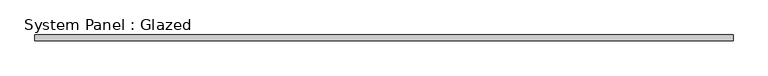
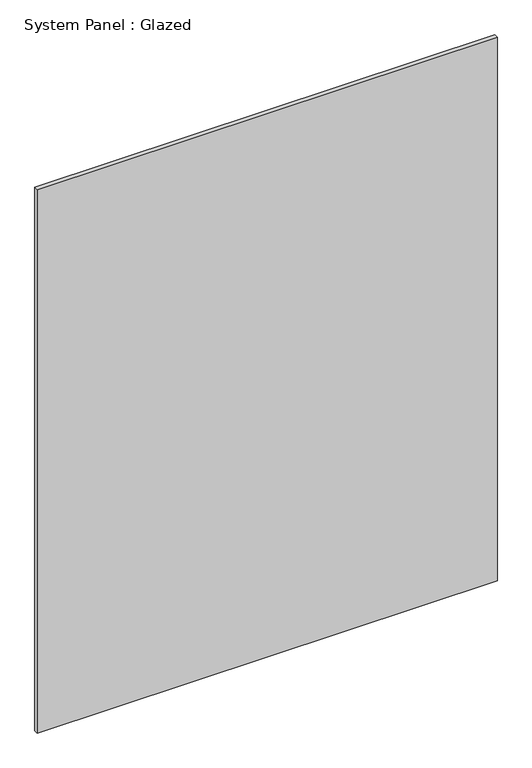
"""IFC4 building model written with IfcOpenShell, lengths in millimetres: plate geometry, System Panel : Glazed."""

from ifc_helpers import new_model, si_unit, origin, origin_with_axes, place, context, project, spatial, polyline, outline, extrude, source, transform, mapped, element, save


def system_panel_glazed_285d4db3(model_context):
    return source(origin(), model_context, "Body", "SweptSolid", [
        extrude(outline(polyline([(1536.7, 19.05), (-1536.7, 19.05), (-1536.7, 44.45), (1536.7, 44.45), (1536.7, 19.05)])), origin_with_axes(), (0.0, 0.0, 1.0), 3835.4),
    ])


if __name__ == "__main__":
    model = new_model("IFC4")
    model_context = context("Model", 3, world=origin())
    ifc_project = project(units=[si_unit("LENGTHUNIT", "METRE", prefix="MILLI")], contexts=[model_context])
    site = spatial("IfcSite", under=ifc_project)
    building = spatial("IfcBuilding", under=site)
    placement = place(None, origin())
    system_panel_glazed_shape = system_panel_glazed_285d4db3(model_context)
    element("IfcPlate", 1, ObjectType="System Panel : Glazed", at=placement, inside=building, context=model_context, shape_type="MappedRepresentation", body=[
        mapped(system_panel_glazed_shape, transform((0.0, 0.0, 0.0), x_axis=(1.0, 0.0, 0.0), y_axis=(0.0, 1.0, 0.0), z_axis=(0.0, 0.0, 1.0))),
    ])
    save(model, "model.ifc")

# Revit data of these elements
# Type "System Panel : Glazed"
#   Construction Type Id = "GSP4R"
#   Analytic Construction = "1/8 in Pilkington single glazing"
#   Visual Light Transmittance = 0.9
#   Solar Heat Gain Coefficient = 0.86
#   Heat Transfer Coefficient (U) = 1.18115 BTU/(h·ft²·°F)
# Element 1 (IfcPlate, "System Panel : Glazed")
#   Materials on its faces: "Glass"
# Materials
#   "Glass": class "Glass", colour RGB 0 128 192, transparency 0.75, Description = "Soda Lime Glass", Cost = 0
